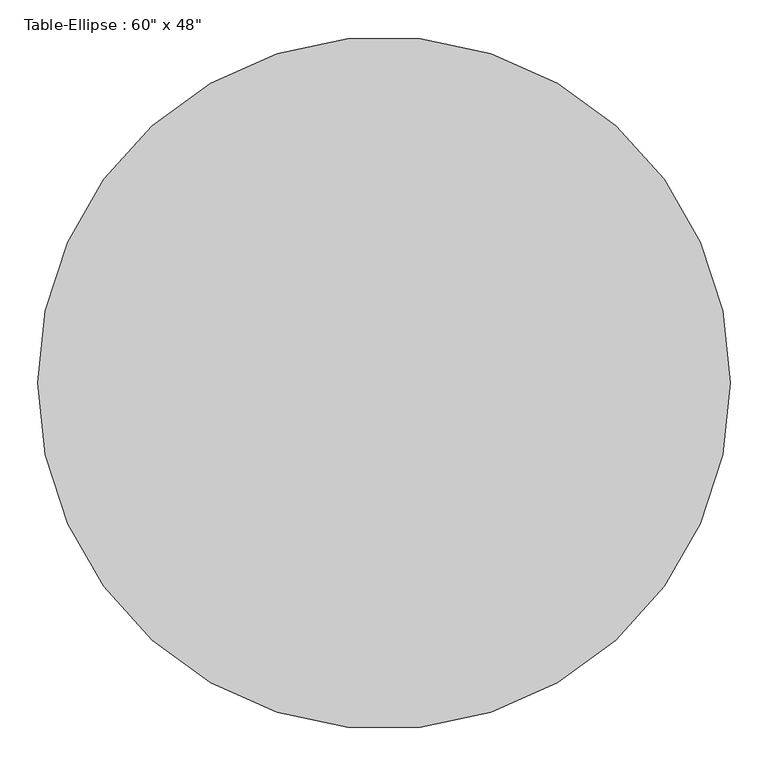
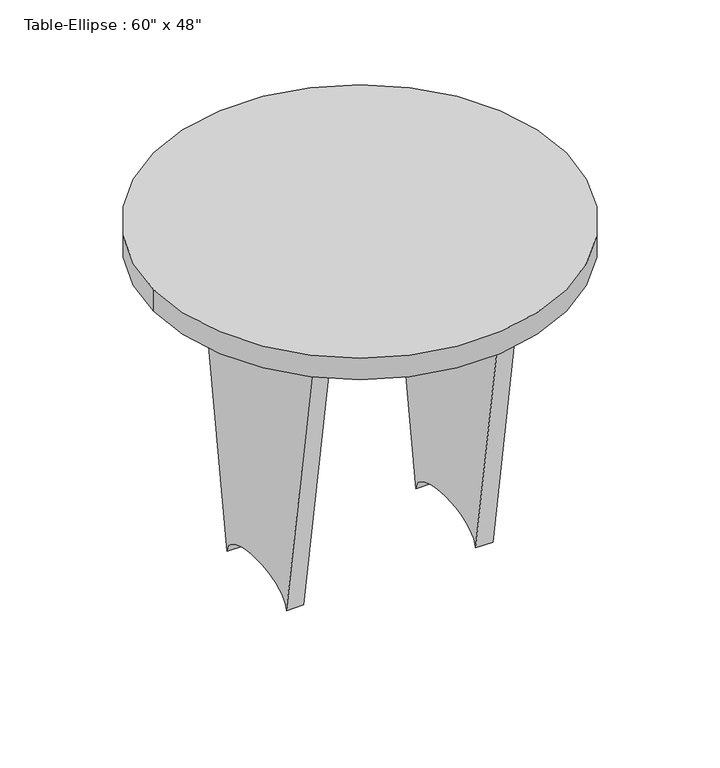
"""IFC4 building model written with IfcOpenShell, lengths in millimetres: furniture geometry."""

from ifc_helpers import new_model, si_unit, point, frame, origin, place, context, project, spatial, circle_curve, ellipse_curve, trimmed, source, transform, mapped, element, save
from ifc_brep_helpers import plane_surface, extruded_surface, advanced_brep


def furniture_4bee3317(model_context):
    return source(origin(), model_context, "Body", "AdvancedBrep", [
        advanced_brep(
        [(-190.5, 19.05, 711.2), (190.5, 19.05, 711.2), (190.5, 19.05, 474.1333333), (-190.5, 19.05, 474.1333333), (-190.5, -19.05, 711.2), (-190.5, -19.05, 474.1333333), (190.5, -19.05, 474.1333333), (190.5, -19.05, 711.2)],
        [
            (0, 1),
            (1, 2),
            (2, 3, ellipse_curve(frame((0.0, 19.05, 474.1333333), z_axis=(0.0, -1.0, 0.0), x_axis=(1.0, 0.0, 0.0)), 190.5, 101.6)),
            (3, 0),
            (4, 5),
            (5, 6, ellipse_curve(frame((0.0, -19.05, 474.1333333), z_axis=(0.0, 1.0, 0.0), x_axis=(1.0, 0.0, 0.0)), 190.5, 101.6)),
            (6, 7),
            (7, 4),
            (0, 4),
            (7, 1),
            (6, 2),
            (5, 3),
        ],
        [
            plane_surface(frame((-190.5, 19.05, 711.2), z_axis=(0.0, 1.0, 0.0), x_axis=(1.0, 0.0, 0.0))),
            plane_surface(frame((-190.5, -19.05, 711.2), z_axis=(0.0, -1.0, 0.0), x_axis=(-1.0, 0.0, 0.0))),
            plane_surface(frame((-190.5, 19.05, 711.2), z_axis=(0.0, 0.0, 1.0), x_axis=(0.0, -1.0, 0.0))),
            plane_surface(frame((190.5, 19.05, 711.2), z_axis=(1.0, 0.0, 0.0), x_axis=(0.0, -1.0, 0.0))),
            extruded_surface(trimmed(ellipse_curve(frame((0.0, -57.15, 474.1333333), z_axis=(0.0, -1.0, 0.0), x_axis=(1.0, 0.0, 0.0)), 190.5, 101.6), [point((190.5, -57.15, 474.1333333))], [point((-190.5, -57.15, 474.1333333))], True, "CARTESIAN"), (0.0, 38.099999999999994, 0.0), 38.099999999999994),
            plane_surface(frame((-190.5, 19.05, 474.1333333), z_axis=(-1.0, 0.0, 0.0), x_axis=(0.0, -1.0, 0.0))),
        ],
        [
            (0, [[1, 2, 3, 4]]),
            (1, [[5, 6, 7, 8]]),
            (2, [[-1, 9, -8, 10]]),
            (3, [[-2, -10, -7, 11]]),
            (4, [[-3, -11, -6, 12]]),
            (5, [[-4, -12, -5, -9]]),
        ],
    ),
        advanced_brep(
        [(228.6, 228.6, 711.2), (228.6, -228.6, 711.2), (228.6, -114.3, 0.0), (228.6, 114.3, 0.0), (190.5, 228.6, 711.2), (190.5, 114.3, 0.0), (190.5, -114.3, 0.0), (190.5, -228.6, 711.2)],
        [
            (0, 1),
            (1, 2),
            (2, 3, ellipse_curve(frame((228.6, 0.0, 0.0), z_axis=(-1.0, 0.0, 0.0), x_axis=(0.0, 1.0, 0.0)), 114.3, 50.8)),
            (3, 0),
            (4, 5),
            (5, 6, ellipse_curve(frame((190.5, 0.0, 0.0), z_axis=(1.0, 0.0, 0.0), x_axis=(0.0, 1.0, 0.0)), 114.3, 50.8)),
            (6, 7),
            (7, 4),
            (0, 4),
            (7, 1),
            (6, 2),
            (5, 3),
        ],
        [
            plane_surface(frame((228.6, -228.6, 711.2), z_axis=(1.0, 0.0, 0.0), x_axis=(0.0, -1.0, 0.0))),
            plane_surface(frame((190.5, -228.6, 711.2), z_axis=(-1.0, 0.0, 0.0), x_axis=(0.0, 1.0, 0.0))),
            plane_surface(frame((228.6, 228.6, 711.2), z_axis=(0.0, 0.0, 1.0), x_axis=(-1.0, 0.0, 0.0))),
            plane_surface(frame((228.6, -228.6, 711.2), z_axis=(0.0, -0.9873303712766982, -0.158678095383759), x_axis=(-1.0, 0.0, 0.0))),
            extruded_surface(trimmed(ellipse_curve(frame((152.4, 0.0, 0.0), z_axis=(-1.0, 0.0, 0.0), x_axis=(0.0, 1.0, 0.0)), 114.3, 50.8), [point((152.4, -114.3, 0.0))], [point((152.4, 114.3, 0.0))], True, "CARTESIAN"), (38.099999999999994, 0.0, 0.0), 38.099999999999994),
            plane_surface(frame((228.6, 114.3, 0.0), z_axis=(0.0, 0.9873303712767002, -0.15867809538374666), x_axis=(-1.0, 0.0, 0.0))),
        ],
        [
            (0, [[1, 2, 3, 4]]),
            (1, [[5, 6, 7, 8]]),
            (2, [[-1, 9, -8, 10]]),
            (3, [[-2, -10, -7, 11]]),
            (4, [[-3, -11, -6, 12]]),
            (5, [[-4, -12, -5, -9]]),
        ],
    ),
        advanced_brep(
        [(-190.5, 228.6, 711.2), (-190.5, -228.6, 711.2), (-190.5, -114.3, 0.0), (-190.5, 114.3, 0.0), (-228.6, 228.6, 711.2), (-228.6, 114.3, 0.0), (-228.6, -114.3, 0.0), (-228.6, -228.6, 711.2)],
        [
            (0, 1),
            (1, 2),
            (2, 3, ellipse_curve(frame((-190.5, 0.0, 0.0), z_axis=(-1.0, 0.0, 0.0), x_axis=(0.0, 1.0, 0.0)), 114.3, 50.8)),
            (3, 0),
            (4, 5),
            (5, 6, ellipse_curve(frame((-228.6, 0.0, 0.0), z_axis=(1.0, 0.0, 0.0), x_axis=(0.0, 1.0, 0.0)), 114.3, 50.8)),
            (6, 7),
            (7, 4),
            (0, 4),
            (7, 1),
            (6, 2),
            (5, 3),
        ],
        [
            plane_surface(frame((-190.5, -228.6, 711.2), z_axis=(1.0, 0.0, 0.0), x_axis=(0.0, -1.0, 0.0))),
            plane_surface(frame((-228.6, -228.6, 711.2), z_axis=(-1.0, 0.0, 0.0), x_axis=(0.0, 1.0, 0.0))),
            plane_surface(frame((-190.5, 228.6, 711.2), z_axis=(0.0, 0.0, 1.0), x_axis=(-1.0, 0.0, 0.0))),
            plane_surface(frame((-190.5, -228.6, 711.2), z_axis=(0.0, -0.9873303712766983, -0.15867809538375854), x_axis=(-1.0, 0.0, 0.0))),
            extruded_surface(trimmed(ellipse_curve(frame((-266.7, 0.0, 0.0), z_axis=(-1.0, 0.0, 0.0), x_axis=(0.0, 1.0, 0.0)), 114.3, 50.8), [point((-266.7, -114.3, 0.0))], [point((-266.7, 114.3, 0.0))], True, "CARTESIAN"), (38.099999999999994, 0.0, 0.0), 38.099999999999994),
            plane_surface(frame((-190.5, 114.3, 0.0), z_axis=(0.0, 0.9873303712766998, -0.15867809538374977), x_axis=(-1.0, 0.0, 0.0))),
        ],
        [
            (0, [[1, 2, 3, 4]]),
            (1, [[5, 6, 7, 8]]),
            (2, [[-1, 9, -8, 10]]),
            (3, [[-2, -10, -7, 11]]),
            (4, [[-3, -11, -6, 12]]),
            (5, [[-4, -12, -5, -9]]),
        ],
    ),
        advanced_brep(
        [(-457.2, 0.0, 762.0), (457.2, 0.0, 762.0), (-457.2, 0.0, 711.2), (457.2, 0.0, 711.2)],
        [
            (0, 1, circle_curve(frame((0.0, 0.0, 762.0), z_axis=(0.0, 0.0, 1.0), x_axis=(1.0, 0.0, 0.0)), 457.2)),
            (1, 0, circle_curve(frame((0.0, 0.0, 762.0), z_axis=(0.0, 0.0, 1.0), x_axis=(1.0, 0.0, 0.0)), 457.2)),
            (2, 3, ellipse_curve(frame((0.0, 0.0, 711.2), z_axis=(0.0, 0.0, -1.0), x_axis=(1.0, 0.0, 0.0)), 457.2, 457.2)),
            (3, 2, ellipse_curve(frame((0.0, 0.0, 711.2), z_axis=(0.0, 0.0, -1.0), x_axis=(1.0, 0.0, 0.0)), 457.2, 457.2)),
            (0, 2),
            (3, 1),
        ],
        [
            plane_surface(frame((457.2, 0.0, 762.0), z_axis=(0.0, 0.0, 1.0), x_axis=(0.0, 1.0, 0.0))),
            plane_surface(frame((457.2, 0.0, 711.2), z_axis=(0.0, 0.0, -1.0), x_axis=(0.0, -1.0, 0.0))),
            extruded_surface(trimmed(ellipse_curve(frame((0.0, 0.0, 660.4), z_axis=(0.0, 0.0, 1.0), x_axis=(1.0, 0.0, 0.0)), 457.2, 457.2), [point((-457.2, 0.0, 660.4))], [point((457.2, 0.0, 660.4))], True, "CARTESIAN"), (0.0, 0.0, 50.80000000000007), 50.80000000000007),
            extruded_surface(trimmed(ellipse_curve(frame((0.0, 0.0, 660.4), z_axis=(0.0, 0.0, 1.0), x_axis=(1.0, 0.0, 0.0)), 457.2, 457.2), [point((457.2, 0.0, 660.4))], [point((-457.2, 0.0, 660.4))], True, "CARTESIAN"), (0.0, 0.0, 50.80000000000007), 50.80000000000007),
        ],
        [
            (0, [[1, 2]]),
            (1, [[3, 4]]),
            (2, [[-1, 5, -4, 6]]),
            (3, [[-2, -6, -3, -5]]),
        ],
    ),
    ])


if __name__ == "__main__":
    model = new_model("IFC4")
    model_context = context("Model", 3, world=origin())
    ifc_project = project(units=[si_unit("LENGTHUNIT", "METRE", prefix="MILLI")], contexts=[model_context])
    site = spatial("IfcSite", under=ifc_project)
    building = spatial("IfcBuilding", under=site)
    placement = place(None, origin())
    furniture_shape = furniture_4bee3317(model_context)
    element("IfcFurniture", 1, ObjectType="Table-Ellipse : 60\" x 48\"", at=placement, inside=building, context=model_context, shape_type="MappedRepresentation", body=[
        mapped(furniture_shape, transform((0.0, 0.0, 0.0), x_axis=(1.0, 0.0, 0.0), y_axis=(0.0, 1.0, 0.0), z_axis=(0.0, 0.0, 1.0))),
    ])
    save(model, "model.ifc")

# Revit data of these elements
# Type "Table-Ellipse : 60\" x 48\""
#   Assembly Code = "E2020200"
#   Half Width = 1' - 6"
#   Half Length = 1' - 6"
#   Height = 2' - 6"
#   Length = 3' - 0"
#   Width = 3' - 0"
#   Base Material = Birch
#   Top Material = Birch
#   Default Elevation = 0
# Element 1 (IfcFurniture, "Table-Ellipse : 60\" x 48\"")
#   Materials on its faces: "Birch"
# Materials
#   "Birch": class "Wood", colour RGB 224 178 126, transparency 0, Description = "Betula Alleghaniensis", Cost = 0
